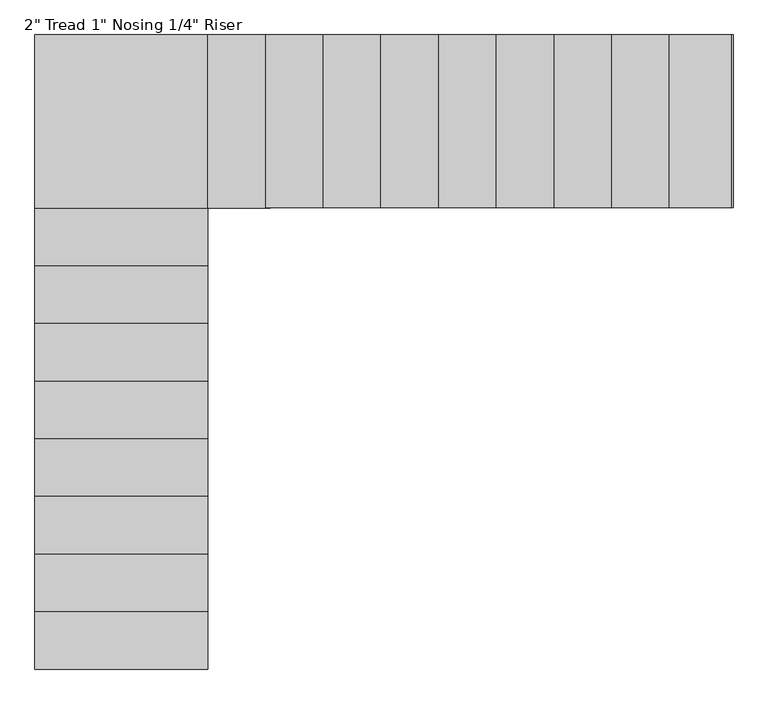
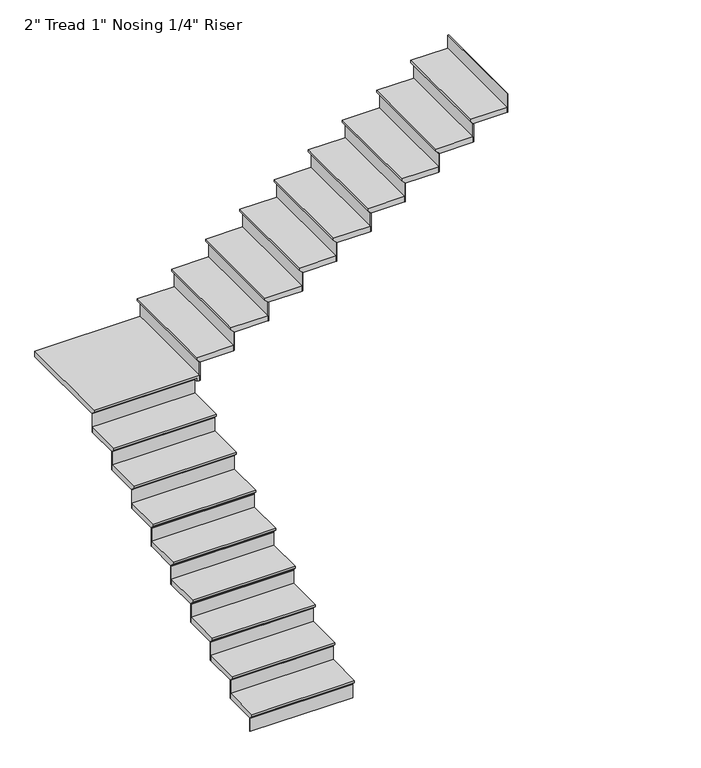
"""IFC4 building model written with IfcOpenShell, lengths in millimetres: stair flight geometry."""

from ifc_helpers import new_model, si_unit, origin, place, context, project, spatial, faceted_brep, source, transform, mapped, element, save


def stair_flight_5496a8fe(model_context):
    return source(origin(), model_context, "Body", "Brep", [
        faceted_brep([(-6027.2757327, 1771.427543, 459.9214286), (-6027.2757327, 1771.427543, 478.9714286), (-6941.6757327, 1771.427543, 478.9714286), (-6941.6757327, 1771.427543, 459.9214286), (-6027.2757327, 1796.827543, 434.5214286), (-6941.6757327, 1796.827543, 434.5214286), (-6027.2757327, 2101.627543, 478.9714286), (-6941.6757327, 2101.627543, 478.9714286), (-6941.6757327, 1796.827543, 428.1714286), (-6941.6757327, 2101.627543, 428.1714286), (-6027.2757327, 2101.627543, 428.1714286), (-6027.2757327, 1796.827543, 428.1714286)], [[[0, 1, 2, 3]], [[4, 0, 3, 5]], [[2, 1, 6, 7]], [[8, 9, 10, 11]], [[2, 7, 9, 8, 5, 3]], [[8, 11, 4, 5]], [[6, 1, 0, 4, 11, 10]], [[7, 6, 10, 9]]]),
        faceted_brep([(-6027.2757327, 1796.827543, 428.1714286), (-6027.2757327, 1796.827543, 304.8), (-6027.2757327, 1803.177543, 304.8), (-6027.2757327, 1803.177543, 428.1714286), (-6941.6757327, 1796.827543, 428.1714286), (-6941.6757327, 1803.177543, 428.1714286), (-6941.6757327, 1803.177543, 304.8), (-6941.6757327, 1796.827543, 304.8)], [[[0, 1, 2, 3]], [[4, 5, 6, 7]], [[1, 0, 4, 7]], [[2, 1, 7, 6]], [[3, 2, 6, 5]], [[0, 3, 5, 4]]]),
        faceted_brep([(-6027.2757327, 2101.627543, 602.3428571), (-6027.2757327, 2101.627543, 428.1714286), (-6027.2757327, 2107.977543, 428.1714286), (-6027.2757327, 2107.977543, 602.3428571), (-6941.6757327, 2101.627543, 602.3428571), (-6941.6757327, 2107.977543, 602.3428571), (-6941.6757327, 2107.977543, 428.1714286), (-6941.6757327, 2101.627543, 428.1714286)], [[[0, 1, 2, 3]], [[4, 5, 6, 7]], [[1, 0, 4, 7]], [[2, 1, 7, 6]], [[3, 2, 6, 5]], [[0, 3, 5, 4]]]),
        faceted_brep([(-6941.6757327, 2076.227543, 653.1428571), (-6027.2757327, 2076.227543, 653.1428571), (-6027.2757327, 2406.427543, 653.1428571), (-6941.6757327, 2406.427543, 653.1428571), (-6941.6757327, 2101.627543, 602.3428571), (-6941.6757327, 2406.427543, 602.3428571), (-6027.2757327, 2406.427543, 602.3428571), (-6027.2757327, 2101.627543, 602.3428571), (-6941.6757327, 2101.627543, 608.6928571), (-6941.6757327, 2076.227543, 634.0928571), (-6027.2757327, 2101.627543, 608.6928571), (-6027.2757327, 2076.227543, 634.0928571)], [[[0, 1, 2, 3]], [[4, 5, 6, 7]], [[0, 3, 5, 4, 8, 9]], [[4, 7, 10, 8]], [[2, 1, 11, 10, 7, 6]], [[3, 2, 6, 5]], [[11, 1, 0, 9]], [[10, 11, 9, 8]]]),
        faceted_brep([(-6027.2757327, 2406.427543, 776.5142857), (-6027.2757327, 2406.427543, 602.3428571), (-6027.2757327, 2412.777543, 602.3428571), (-6027.2757327, 2412.777543, 776.5142857), (-6941.6757327, 2406.427543, 776.5142857), (-6941.6757327, 2412.777543, 776.5142857), (-6941.6757327, 2412.777543, 602.3428571), (-6941.6757327, 2406.427543, 602.3428571)], [[[0, 1, 2, 3]], [[4, 5, 6, 7]], [[1, 0, 4, 7]], [[2, 1, 7, 6]], [[3, 2, 6, 5]], [[0, 3, 5, 4]]]),
        faceted_brep([(-6941.6757327, 2381.027543, 827.3142857), (-6027.2757327, 2381.027543, 827.3142857), (-6027.2757327, 2711.227543, 827.3142857), (-6941.6757327, 2711.227543, 827.3142857), (-6941.6757327, 2406.427543, 776.5142857), (-6941.6757327, 2711.227543, 776.5142857), (-6027.2757327, 2711.227543, 776.5142857), (-6027.2757327, 2406.427543, 776.5142857), (-6941.6757327, 2406.427543, 782.8642857), (-6941.6757327, 2381.027543, 808.2642857), (-6027.2757327, 2406.427543, 782.8642857), (-6027.2757327, 2381.027543, 808.2642857)], [[[0, 1, 2, 3]], [[4, 5, 6, 7]], [[0, 3, 5, 4, 8, 9]], [[4, 7, 10, 8]], [[2, 1, 11, 10, 7, 6]], [[3, 2, 6, 5]], [[11, 1, 0, 9]], [[10, 11, 9, 8]]]),
        faceted_brep([(-6027.2757327, 2711.227543, 950.6857143), (-6027.2757327, 2711.227543, 776.5142857), (-6027.2757327, 2717.577543, 776.5142857), (-6027.2757327, 2717.577543, 950.6857143), (-6941.6757327, 2711.227543, 950.6857143), (-6941.6757327, 2717.577543, 950.6857143), (-6941.6757327, 2717.577543, 776.5142857), (-6941.6757327, 2711.227543, 776.5142857)], [[[0, 1, 2, 3]], [[4, 5, 6, 7]], [[1, 0, 4, 7]], [[2, 1, 7, 6]], [[3, 2, 6, 5]], [[0, 3, 5, 4]]]),
        faceted_brep([(-6941.6757327, 2685.827543, 1001.4857143), (-6027.2757327, 2685.827543, 1001.4857143), (-6027.2757327, 3016.027543, 1001.4857143), (-6941.6757327, 3016.027543, 1001.4857143), (-6941.6757327, 2711.227543, 950.6857143), (-6941.6757327, 3016.027543, 950.6857143), (-6027.2757327, 3016.027543, 950.6857143), (-6027.2757327, 2711.227543, 950.6857143), (-6941.6757327, 2711.227543, 957.0357143), (-6941.6757327, 2685.827543, 982.4357143), (-6027.2757327, 2711.227543, 957.0357143), (-6027.2757327, 2685.827543, 982.4357143)], [[[0, 1, 2, 3]], [[4, 5, 6, 7]], [[0, 3, 5, 4, 8, 9]], [[4, 7, 10, 8]], [[2, 1, 11, 10, 7, 6]], [[3, 2, 6, 5]], [[11, 1, 0, 9]], [[10, 11, 9, 8]]]),
        faceted_brep([(-6027.2757327, 3016.027543, 1124.8571429), (-6027.2757327, 3016.027543, 950.6857143), (-6027.2757327, 3022.377543, 950.6857143), (-6027.2757327, 3022.377543, 1124.8571429), (-6941.6757327, 3016.027543, 1124.8571429), (-6941.6757327, 3022.377543, 1124.8571429), (-6941.6757327, 3022.377543, 950.6857143), (-6941.6757327, 3016.027543, 950.6857143)], [[[0, 1, 2, 3]], [[4, 5, 6, 7]], [[1, 0, 4, 7]], [[2, 1, 7, 6]], [[3, 2, 6, 5]], [[0, 3, 5, 4]]]),
        faceted_brep([(-6941.6757327, 2990.627543, 1175.6571429), (-6027.2757327, 2990.627543, 1175.6571429), (-6027.2757327, 3320.827543, 1175.6571429), (-6941.6757327, 3320.827543, 1175.6571429), (-6941.6757327, 3016.027543, 1124.8571429), (-6941.6757327, 3320.827543, 1124.8571429), (-6027.2757327, 3320.827543, 1124.8571429), (-6027.2757327, 3016.027543, 1124.8571429), (-6941.6757327, 3016.027543, 1131.2071429), (-6941.6757327, 2990.627543, 1156.6071429), (-6027.2757327, 3016.027543, 1131.2071429), (-6027.2757327, 2990.627543, 1156.6071429)], [[[0, 1, 2, 3]], [[4, 5, 6, 7]], [[0, 3, 5, 4, 8, 9]], [[4, 7, 10, 8]], [[2, 1, 11, 10, 7, 6]], [[3, 2, 6, 5]], [[11, 1, 0, 9]], [[10, 11, 9, 8]]]),
        faceted_brep([(-6027.2757327, 3320.827543, 1299.0285714), (-6027.2757327, 3320.827543, 1124.8571429), (-6027.2757327, 3327.177543, 1124.8571429), (-6027.2757327, 3327.177543, 1299.0285714), (-6941.6757327, 3320.827543, 1299.0285714), (-6941.6757327, 3327.177543, 1299.0285714), (-6941.6757327, 3327.177543, 1124.8571429), (-6941.6757327, 3320.827543, 1124.8571429)], [[[0, 1, 2, 3]], [[4, 5, 6, 7]], [[1, 0, 4, 7]], [[2, 1, 7, 6]], [[3, 2, 6, 5]], [[0, 3, 5, 4]]]),
        faceted_brep([(-6941.6757327, 3295.427543, 1349.8285714), (-6027.2757327, 3295.427543, 1349.8285714), (-6027.2757327, 3625.627543, 1349.8285714), (-6941.6757327, 3625.627543, 1349.8285714), (-6941.6757327, 3320.827543, 1299.0285714), (-6941.6757327, 3625.627543, 1299.0285714), (-6027.2757327, 3625.627543, 1299.0285714), (-6027.2757327, 3320.827543, 1299.0285714), (-6941.6757327, 3320.827543, 1305.3785714), (-6941.6757327, 3295.427543, 1330.7785714), (-6027.2757327, 3320.827543, 1305.3785714), (-6027.2757327, 3295.427543, 1330.7785714)], [[[0, 1, 2, 3]], [[4, 5, 6, 7]], [[0, 3, 5, 4, 8, 9]], [[4, 7, 10, 8]], [[2, 1, 11, 10, 7, 6]], [[3, 2, 6, 5]], [[11, 1, 0, 9]], [[10, 11, 9, 8]]]),
        faceted_brep([(-6027.2757327, 3625.627543, 1473.2), (-6027.2757327, 3625.627543, 1299.0285714), (-6027.2757327, 3631.977543, 1299.0285714), (-6027.2757327, 3631.977543, 1473.2), (-6941.6757327, 3625.627543, 1473.2), (-6941.6757327, 3631.977543, 1473.2), (-6941.6757327, 3631.977543, 1299.0285714), (-6941.6757327, 3625.627543, 1299.0285714)], [[[0, 1, 2, 3]], [[4, 5, 6, 7]], [[1, 0, 4, 7]], [[2, 1, 7, 6]], [[3, 2, 6, 5]], [[0, 3, 5, 4]]]),
        faceted_brep([(-6941.6757327, 3600.227543, 1524.0), (-6027.2757327, 3600.227543, 1524.0), (-6027.2757327, 3930.427543, 1524.0), (-6941.6757327, 3930.427543, 1524.0), (-6941.6757327, 3625.627543, 1473.2), (-6941.6757327, 3930.427543, 1473.2), (-6027.2757327, 3930.427543, 1473.2), (-6027.2757327, 3625.627543, 1473.2), (-6941.6757327, 3625.627543, 1479.55), (-6941.6757327, 3600.227543, 1504.95), (-6027.2757327, 3625.627543, 1479.55), (-6027.2757327, 3600.227543, 1504.95)], [[[0, 1, 2, 3]], [[4, 5, 6, 7]], [[0, 3, 5, 4, 8, 9]], [[4, 7, 10, 8]], [[2, 1, 11, 10, 7, 6]], [[3, 2, 6, 5]], [[11, 1, 0, 9]], [[10, 11, 9, 8]]]),
        faceted_brep([(-6027.2757327, 3930.427543, 1647.3714286), (-6027.2757327, 3930.427543, 1473.2), (-6027.2757327, 3936.777543, 1473.2), (-6027.2757327, 3936.777543, 1647.3714286), (-6941.6757327, 3930.427543, 1647.3714286), (-6941.6757327, 3936.777543, 1647.3714286), (-6941.6757327, 3936.777543, 1473.2), (-6941.6757327, 3930.427543, 1473.2)], [[[0, 1, 2, 3]], [[4, 5, 6, 7]], [[1, 0, 4, 7]], [[2, 1, 7, 6]], [[3, 2, 6, 5]], [[0, 3, 5, 4]]]),
        faceted_brep([(-6941.6757327, 3905.027543, 1698.1714286), (-6027.2757327, 3905.027543, 1698.1714286), (-6027.2757327, 4235.227543, 1698.1714286), (-6941.6757327, 4235.227543, 1698.1714286), (-6941.6757327, 3930.427543, 1647.3714286), (-6941.6757327, 4235.227543, 1647.3714286), (-6027.2757327, 4235.227543, 1647.3714286), (-6027.2757327, 3930.427543, 1647.3714286), (-6941.6757327, 3930.427543, 1653.7214286), (-6941.6757327, 3905.027543, 1679.1214286), (-6027.2757327, 3930.427543, 1653.7214286), (-6027.2757327, 3905.027543, 1679.1214286)], [[[0, 1, 2, 3]], [[4, 5, 6, 7]], [[0, 3, 5, 4, 8, 9]], [[4, 7, 10, 8]], [[2, 1, 11, 10, 7, 6]], [[3, 2, 6, 5]], [[11, 1, 0, 9]], [[10, 11, 9, 8]]]),
        faceted_brep([(-6027.2757327, 4235.227543, 1821.5428571), (-6027.2757327, 4235.227543, 1647.3714286), (-6027.2757327, 4241.577543, 1647.3714286), (-6027.2757327, 4241.577543, 1821.5428571), (-6941.6757327, 4235.227543, 1821.5428571), (-6941.6757327, 4241.577543, 1821.5428571), (-6941.6757327, 4241.577543, 1647.3714286), (-6941.6757327, 4235.227543, 1647.3714286)], [[[0, 1, 2, 3]], [[4, 5, 6, 7]], [[1, 0, 4, 7]], [[2, 1, 7, 6]], [[3, 2, 6, 5]], [[0, 3, 5, 4]]]),
        faceted_brep([(-6001.8757327, 5124.227543, 1872.3428571), (-6941.6757327, 5124.227543, 1872.3428571), (-6941.6757327, 4209.827543, 1872.3428571), (-6001.8757327, 4209.827543, 1872.3428571), (-6941.6757327, 5124.227543, 1821.5428571), (-6001.8757327, 5124.227543, 1821.5428571), (-6001.8757327, 4209.827543, 1821.5428571), (-6027.2757327, 4209.827543, 1821.5428571), (-6027.2757327, 4235.227543, 1821.5428571), (-6941.6757327, 4235.227543, 1821.5428571), (-6941.6757327, 4235.227543, 1827.8928571), (-6941.6757327, 4209.827543, 1853.2928571), (-6027.2757327, 4235.227543, 1827.8928571), (-6027.2757327, 4209.827543, 1853.2928571)], [[[0, 1, 2, 3]], [[4, 5, 6, 7, 8, 9]], [[1, 0, 5, 4]], [[2, 1, 4, 9, 10, 11]], [[9, 8, 12, 10]], [[8, 7, 13, 12]], [[3, 2, 11, 13, 7, 6]], [[0, 3, 6, 5]], [[11, 10, 12, 13]]]),
        faceted_brep([(-6001.8757327, 4209.827543, 1995.7142857), (-6001.8757327, 4209.827543, 1821.5428571), (-5995.5257327, 4209.827543, 1821.5428571), (-5995.5257327, 4209.827543, 1995.7142857), (-6001.8757327, 5124.227543, 1995.7142857), (-5995.5257327, 5124.227543, 1995.7142857), (-5995.5257327, 5124.227543, 1821.5428571), (-6001.8757327, 5124.227543, 1821.5428571)], [[[0, 1, 2, 3]], [[4, 5, 6, 7]], [[1, 0, 4, 7]], [[2, 1, 7, 6]], [[3, 2, 6, 5]], [[0, 3, 5, 4]]]),
        faceted_brep([(-6027.2757327, 5124.227543, 2046.5142857), (-6027.2757327, 4209.827543, 2046.5142857), (-5697.0757327, 4209.827543, 2046.5142857), (-5697.0757327, 5124.227543, 2046.5142857), (-6001.8757327, 5124.227543, 1995.7142857), (-5697.0757327, 5124.227543, 1995.7142857), (-5697.0757327, 4209.827543, 1995.7142857), (-6001.8757327, 4209.827543, 1995.7142857), (-6001.8757327, 5124.227543, 2002.0642857), (-6027.2757327, 5124.227543, 2027.4642857), (-6001.8757327, 4209.827543, 2002.0642857), (-6027.2757327, 4209.827543, 2027.4642857)], [[[0, 1, 2, 3]], [[4, 5, 6, 7]], [[0, 3, 5, 4, 8, 9]], [[4, 7, 10, 8]], [[2, 1, 11, 10, 7, 6]], [[3, 2, 6, 5]], [[11, 1, 0, 9]], [[10, 11, 9, 8]]]),
        faceted_brep([(-5697.0757327, 4209.827543, 2169.8857143), (-5697.0757327, 4209.827543, 1995.7142857), (-5690.7257327, 4209.827543, 1995.7142857), (-5690.7257327, 4209.827543, 2169.8857143), (-5697.0757327, 5124.227543, 2169.8857143), (-5690.7257327, 5124.227543, 2169.8857143), (-5690.7257327, 5124.227543, 1995.7142857), (-5697.0757327, 5124.227543, 1995.7142857)], [[[0, 1, 2, 3]], [[4, 5, 6, 7]], [[1, 0, 4, 7]], [[2, 1, 7, 6]], [[3, 2, 6, 5]], [[0, 3, 5, 4]]]),
        faceted_brep([(-5722.4757327, 5124.227543, 2220.6857143), (-5722.4757327, 4209.827543, 2220.6857143), (-5392.2757327, 4209.827543, 2220.6857143), (-5392.2757327, 5124.227543, 2220.6857143), (-5697.0757327, 5124.227543, 2169.8857143), (-5392.2757327, 5124.227543, 2169.8857143), (-5392.2757327, 4209.827543, 2169.8857143), (-5697.0757327, 4209.827543, 2169.8857143), (-5697.0757327, 5124.227543, 2176.2357143), (-5722.4757327, 5124.227543, 2201.6357143), (-5697.0757327, 4209.827543, 2176.2357143), (-5722.4757327, 4209.827543, 2201.6357143)], [[[0, 1, 2, 3]], [[4, 5, 6, 7]], [[0, 3, 5, 4, 8, 9]], [[4, 7, 10, 8]], [[2, 1, 11, 10, 7, 6]], [[3, 2, 6, 5]], [[11, 1, 0, 9]], [[10, 11, 9, 8]]]),
        faceted_brep([(-5392.2757327, 4209.827543, 2344.0571429), (-5392.2757327, 4209.827543, 2169.8857143), (-5385.9257327, 4209.827543, 2169.8857143), (-5385.9257327, 4209.827543, 2344.0571429), (-5392.2757327, 5124.227543, 2344.0571429), (-5385.9257327, 5124.227543, 2344.0571429), (-5385.9257327, 5124.227543, 2169.8857143), (-5392.2757327, 5124.227543, 2169.8857143)], [[[0, 1, 2, 3]], [[4, 5, 6, 7]], [[1, 0, 4, 7]], [[2, 1, 7, 6]], [[3, 2, 6, 5]], [[0, 3, 5, 4]]]),
        faceted_brep([(-5417.6757327, 5124.227543, 2394.8571429), (-5417.6757327, 4209.827543, 2394.8571429), (-5087.4757327, 4209.827543, 2394.8571429), (-5087.4757327, 5124.227543, 2394.8571429), (-5392.2757327, 5124.227543, 2344.0571429), (-5087.4757327, 5124.227543, 2344.0571429), (-5087.4757327, 4209.827543, 2344.0571429), (-5392.2757327, 4209.827543, 2344.0571429), (-5392.2757327, 5124.227543, 2350.4071429), (-5417.6757327, 5124.227543, 2375.8071429), (-5392.2757327, 4209.827543, 2350.4071429), (-5417.6757327, 4209.827543, 2375.8071429)], [[[0, 1, 2, 3]], [[4, 5, 6, 7]], [[0, 3, 5, 4, 8, 9]], [[4, 7, 10, 8]], [[2, 1, 11, 10, 7, 6]], [[3, 2, 6, 5]], [[11, 1, 0, 9]], [[10, 11, 9, 8]]]),
        faceted_brep([(-5087.4757327, 4209.827543, 2518.2285714), (-5087.4757327, 4209.827543, 2344.0571429), (-5081.1257327, 4209.827543, 2344.0571429), (-5081.1257327, 4209.827543, 2518.2285714), (-5087.4757327, 5124.227543, 2518.2285714), (-5081.1257327, 5124.227543, 2518.2285714), (-5081.1257327, 5124.227543, 2344.0571429), (-5087.4757327, 5124.227543, 2344.0571429)], [[[0, 1, 2, 3]], [[4, 5, 6, 7]], [[1, 0, 4, 7]], [[2, 1, 7, 6]], [[3, 2, 6, 5]], [[0, 3, 5, 4]]]),
        faceted_brep([(-5112.8757327, 5124.227543, 2569.0285714), (-5112.8757327, 4209.827543, 2569.0285714), (-4782.6757327, 4209.827543, 2569.0285714), (-4782.6757327, 5124.227543, 2569.0285714), (-5087.4757327, 5124.227543, 2518.2285714), (-4782.6757327, 5124.227543, 2518.2285714), (-4782.6757327, 4209.827543, 2518.2285714), (-5087.4757327, 4209.827543, 2518.2285714), (-5087.4757327, 5124.227543, 2524.5785714), (-5112.8757327, 5124.227543, 2549.9785714), (-5087.4757327, 4209.827543, 2524.5785714), (-5112.8757327, 4209.827543, 2549.9785714)], [[[0, 1, 2, 3]], [[4, 5, 6, 7]], [[0, 3, 5, 4, 8, 9]], [[4, 7, 10, 8]], [[2, 1, 11, 10, 7, 6]], [[3, 2, 6, 5]], [[11, 1, 0, 9]], [[10, 11, 9, 8]]]),
        faceted_brep([(-4782.6757327, 4209.827543, 2692.4), (-4782.6757327, 4209.827543, 2518.2285714), (-4776.3257327, 4209.827543, 2518.2285714), (-4776.3257327, 4209.827543, 2692.4), (-4782.6757327, 5124.227543, 2692.4), (-4776.3257327, 5124.227543, 2692.4), (-4776.3257327, 5124.227543, 2518.2285714), (-4782.6757327, 5124.227543, 2518.2285714)], [[[0, 1, 2, 3]], [[4, 5, 6, 7]], [[1, 0, 4, 7]], [[2, 1, 7, 6]], [[3, 2, 6, 5]], [[0, 3, 5, 4]]]),
        faceted_brep([(-4808.0757327, 5124.227543, 2743.2), (-4808.0757327, 4209.827543, 2743.2), (-4477.8757327, 4209.827543, 2743.2), (-4477.8757327, 5124.227543, 2743.2), (-4782.6757327, 5124.227543, 2692.4), (-4477.8757327, 5124.227543, 2692.4), (-4477.8757327, 4209.827543, 2692.4), (-4782.6757327, 4209.827543, 2692.4), (-4782.6757327, 5124.227543, 2698.75), (-4808.0757327, 5124.227543, 2724.15), (-4782.6757327, 4209.827543, 2698.75), (-4808.0757327, 4209.827543, 2724.15)], [[[0, 1, 2, 3]], [[4, 5, 6, 7]], [[0, 3, 5, 4, 8, 9]], [[4, 7, 10, 8]], [[2, 1, 11, 10, 7, 6]], [[3, 2, 6, 5]], [[11, 1, 0, 9]], [[10, 11, 9, 8]]]),
        faceted_brep([(-4477.8757327, 4209.827543, 2866.5714286), (-4477.8757327, 4209.827543, 2692.4), (-4471.5257327, 4209.827543, 2692.4), (-4471.5257327, 4209.827543, 2866.5714286), (-4477.8757327, 5124.227543, 2866.5714286), (-4471.5257327, 5124.227543, 2866.5714286), (-4471.5257327, 5124.227543, 2692.4), (-4477.8757327, 5124.227543, 2692.4)], [[[0, 1, 2, 3]], [[4, 5, 6, 7]], [[1, 0, 4, 7]], [[2, 1, 7, 6]], [[3, 2, 6, 5]], [[0, 3, 5, 4]]]),
        faceted_brep([(-4503.2757327, 5124.227543, 2917.3714286), (-4503.2757327, 4209.827543, 2917.3714286), (-4173.0757327, 4209.827543, 2917.3714286), (-4173.0757327, 5124.227543, 2917.3714286), (-4477.8757327, 5124.227543, 2866.5714286), (-4173.0757327, 5124.227543, 2866.5714286), (-4173.0757327, 4209.827543, 2866.5714286), (-4477.8757327, 4209.827543, 2866.5714286), (-4477.8757327, 5124.227543, 2872.9214286), (-4503.2757327, 5124.227543, 2898.3214286), (-4477.8757327, 4209.827543, 2872.9214286), (-4503.2757327, 4209.827543, 2898.3214286)], [[[0, 1, 2, 3]], [[4, 5, 6, 7]], [[0, 3, 5, 4, 8, 9]], [[4, 7, 10, 8]], [[2, 1, 11, 10, 7, 6]], [[3, 2, 6, 5]], [[11, 1, 0, 9]], [[10, 11, 9, 8]]]),
        faceted_brep([(-4173.0757327, 4209.827543, 3040.7428571), (-4173.0757327, 4209.827543, 2866.5714286), (-4166.7257327, 4209.827543, 2866.5714286), (-4166.7257327, 4209.827543, 3040.7428571), (-4173.0757327, 5124.227543, 3040.7428571), (-4166.7257327, 5124.227543, 3040.7428571), (-4166.7257327, 5124.227543, 2866.5714286), (-4173.0757327, 5124.227543, 2866.5714286)], [[[0, 1, 2, 3]], [[4, 5, 6, 7]], [[1, 0, 4, 7]], [[2, 1, 7, 6]], [[3, 2, 6, 5]], [[0, 3, 5, 4]]]),
        faceted_brep([(-4198.4757327, 5124.227543, 3091.5428571), (-4198.4757327, 4209.827543, 3091.5428571), (-3868.2757327, 4209.827543, 3091.5428571), (-3868.2757327, 5124.227543, 3091.5428571), (-4173.0757327, 5124.227543, 3040.7428571), (-3868.2757327, 5124.227543, 3040.7428571), (-3868.2757327, 4209.827543, 3040.7428571), (-4173.0757327, 4209.827543, 3040.7428571), (-4173.0757327, 5124.227543, 3047.0928571), (-4198.4757327, 5124.227543, 3072.4928571), (-4173.0757327, 4209.827543, 3047.0928571), (-4198.4757327, 4209.827543, 3072.4928571)], [[[0, 1, 2, 3]], [[4, 5, 6, 7]], [[0, 3, 5, 4, 8, 9]], [[4, 7, 10, 8]], [[2, 1, 11, 10, 7, 6]], [[3, 2, 6, 5]], [[11, 1, 0, 9]], [[10, 11, 9, 8]]]),
        faceted_brep([(-3868.2757327, 4209.827543, 3214.9142857), (-3868.2757327, 4209.827543, 3040.7428571), (-3861.9257327, 4209.827543, 3040.7428571), (-3861.9257327, 4209.827543, 3214.9142857), (-3868.2757327, 5124.227543, 3214.9142857), (-3861.9257327, 5124.227543, 3214.9142857), (-3861.9257327, 5124.227543, 3040.7428571), (-3868.2757327, 5124.227543, 3040.7428571)], [[[0, 1, 2, 3]], [[4, 5, 6, 7]], [[1, 0, 4, 7]], [[2, 1, 7, 6]], [[3, 2, 6, 5]], [[0, 3, 5, 4]]]),
        faceted_brep([(-3893.6757327, 5124.227543, 3265.7142857), (-3893.6757327, 4209.827543, 3265.7142857), (-3563.4757327, 4209.827543, 3265.7142857), (-3563.4757327, 5124.227543, 3265.7142857), (-3868.2757327, 5124.227543, 3214.9142857), (-3563.4757327, 5124.227543, 3214.9142857), (-3563.4757327, 4209.827543, 3214.9142857), (-3868.2757327, 4209.827543, 3214.9142857), (-3868.2757327, 5124.227543, 3221.2642857), (-3893.6757327, 5124.227543, 3246.6642857), (-3868.2757327, 4209.827543, 3221.2642857), (-3893.6757327, 4209.827543, 3246.6642857)], [[[0, 1, 2, 3]], [[4, 5, 6, 7]], [[0, 3, 5, 4, 8, 9]], [[4, 7, 10, 8]], [[2, 1, 11, 10, 7, 6]], [[3, 2, 6, 5]], [[11, 1, 0, 9]], [[10, 11, 9, 8]]]),
        faceted_brep([(-3563.4757327, 4209.827543, 3389.0857143), (-3563.4757327, 4209.827543, 3214.9142857), (-3557.1257327, 4209.827543, 3214.9142857), (-3557.1257327, 4209.827543, 3389.0857143), (-3563.4757327, 5124.227543, 3389.0857143), (-3557.1257327, 5124.227543, 3389.0857143), (-3557.1257327, 5124.227543, 3214.9142857), (-3563.4757327, 5124.227543, 3214.9142857)], [[[0, 1, 2, 3]], [[4, 5, 6, 7]], [[1, 0, 4, 7]], [[2, 1, 7, 6]], [[3, 2, 6, 5]], [[0, 3, 5, 4]]]),
        faceted_brep([(-3258.6757327, 4209.827543, 3563.2571429), (-3258.6757327, 4209.827543, 3389.0857143), (-3252.3257327, 4209.827543, 3389.0857143), (-3252.3257327, 4209.827543, 3563.2571429), (-3258.6757327, 5124.227543, 3563.2571429), (-3252.3257327, 5124.227543, 3563.2571429), (-3252.3257327, 5124.227543, 3389.0857143), (-3258.6757327, 5124.227543, 3389.0857143)], [[[0, 1, 2, 3]], [[4, 5, 6, 7]], [[1, 0, 4, 7]], [[2, 1, 7, 6]], [[3, 2, 6, 5]], [[0, 3, 5, 4]]]),
        faceted_brep([(-3588.8757327, 5124.227543, 3439.8857143), (-3588.8757327, 4209.827543, 3439.8857143), (-3258.6757327, 4209.827543, 3439.8857143), (-3258.6757327, 5124.227543, 3439.8857143), (-3563.4757327, 5124.227543, 3389.0857143), (-3258.6757327, 5124.227543, 3389.0857143), (-3258.6757327, 4209.827543, 3389.0857143), (-3563.4757327, 4209.827543, 3389.0857143), (-3563.4757327, 5124.227543, 3395.4357143), (-3588.8757327, 5124.227543, 3420.8357143), (-3563.4757327, 4209.827543, 3395.4357143), (-3588.8757327, 4209.827543, 3420.8357143)], [[[0, 1, 2, 3]], [[4, 5, 6, 7]], [[0, 3, 5, 4, 8, 9]], [[4, 7, 10, 8]], [[2, 1, 11, 10, 7, 6]], [[3, 2, 6, 5]], [[11, 1, 0, 9]], [[10, 11, 9, 8]]]),
    ])


if __name__ == "__main__":
    model = new_model("IFC4")
    model_context = context("Model", 3, world=origin())
    ifc_project = project(units=[si_unit("LENGTHUNIT", "METRE", prefix="MILLI")], contexts=[model_context])
    site = spatial("IfcSite", under=ifc_project)
    building = spatial("IfcBuilding", under=site)
    placement = place(None, origin())
    stair_flight_shape = stair_flight_5496a8fe(model_context)
    element("IfcStairFlight", 1, ObjectType="2\" Tread 1\" Nosing 1/4\" Riser", at=placement, inside=building, context=model_context, shape_type="MappedRepresentation", body=[
        mapped(stair_flight_shape, transform((0.0, 0.0, 0.0), x_axis=(1.0, 0.0, 0.0), y_axis=(0.0, 1.0, 0.0), z_axis=(0.0, 0.0, 1.0))),
    ])
    save(model, "model.ifc")

# Revit data of these elements
# Element 1 (IfcStairFlight, "2\" Tread 1\" Nosing 1/4\" Riser")
#   Materials on its faces: "MARBLE FLOORING"
# Materials
#   "MARBLE FLOORING": class "Generic", colour RGB 120 120 120, transparency 0, Cost = 0
